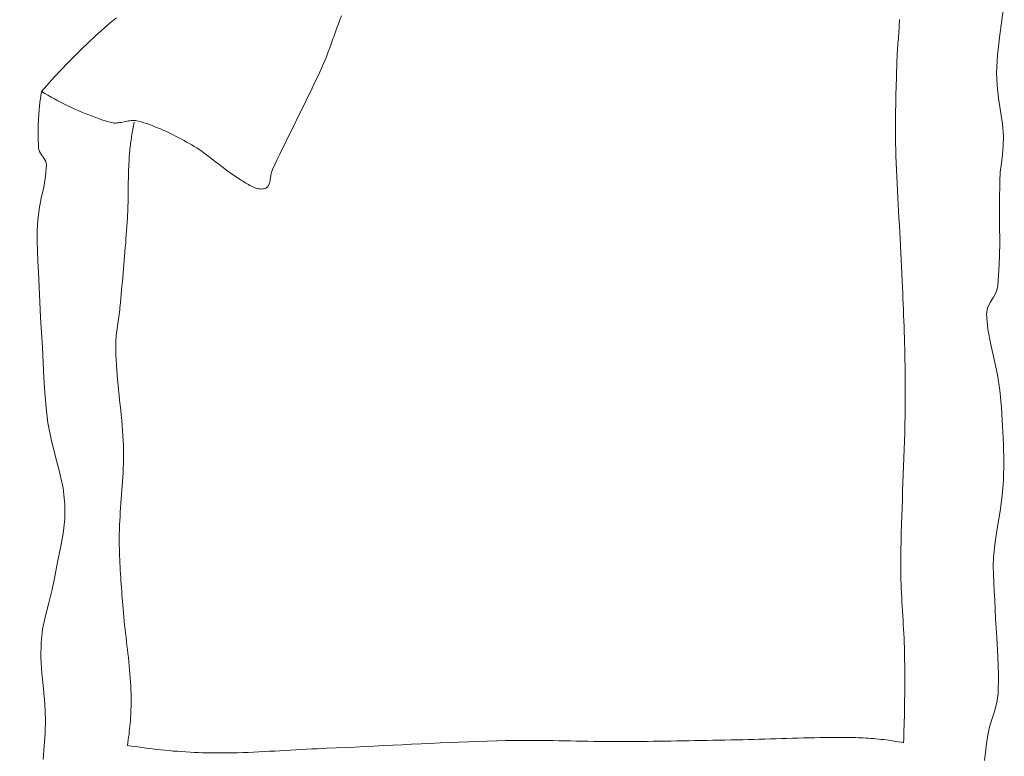
# Model space of a CAD drawing. Units: inches. Extents: x 1484 to 2008, y 1843 to 2590.
# Tile 13 of 21: x 1802 to 1862, y 2126 to 2172. Entities that reach past the tile are written whole.
import ezdxf

# ---------------------------------------------------------------- set-up
doc = ezdxf.new("R2010")
doc.units = ezdxf.units.IN
doc.layers.add('A-ANNO-DIMS', color=2, linetype='Continuous', lineweight=18)
doc.layers.add('A-FURN', color=8, linetype='Continuous', lineweight=18)
doc.styles.get("Standard").update_dxf_attribs({"font": 'arial.ttf'})
doc.dimstyles.new('ISO-25', dxfattribs={"dimtxt": 7, "dimasz": 2.5, "dimexe": 1.25, "dimexo": 0.625, "dimtad": 1, "dimdec": 0, "dimlunit": 3, "dimtxsty": 'Standard', "dimcen": 2.5, "dimadec": 0, "dimazin": 0, "dimtfac": 1, "dimtdec": 0, "dimtmove": 0, "dimatfit": 3, "dimfxl": 1, "dimarcsym": 0})

# ---------------------------------------------------------------- blocks, each defined once
blk = doc.blocks.new('BED-DOUBLE')
for p, q in [((59.548, 52.555), (59.695, 53.637)), ((4.496, 52.387), (3.604, 51.587)), ((4.899, 52.699), (4.496, 52.387)), ((18.499, 52.08), (18.59, 52.327)), ((18.59, 52.327), (18.683, 52.572)), ((18.683, 52.572), (18.778, 52.816)), ((53.205, 52.138), (53.211, 52.285)), ((53.211, 52.285), (53.216, 52.432)), ((53.216, 52.432), (53.22, 52.579)), ((59.397, 51.474), (59.548, 52.555)), ((18.322, 51.584), (18.41, 51.832)), ((18.41, 51.832), (18.499, 52.08)), ((53.167, 51.551), (53.178, 51.698)), ((53.178, 51.698), (53.188, 51.844)), ((53.188, 51.844), (53.197, 51.991)), ((53.197, 51.991), (53.205, 52.138)), ((3.604, 51.587), (2.733, 50.763)), ((18.055, 50.84), (18.145, 51.088)), ((18.145, 51.088), (18.234, 51.336)), ((18.234, 51.336), (18.322, 51.584)), ((53.121, 50.964), (53.133, 51.111)), ((53.133, 51.111), (53.144, 51.257)), ((53.144, 51.257), (53.156, 51.404)), ((53.156, 51.404), (53.167, 51.551)), ((59.275, 50.39), (59.397, 51.474)), ((2.733, 50.763), (1.886, 49.914)), ((17.87, 50.349), (17.964, 50.594)), ((17.964, 50.594), (18.055, 50.84)), ((53.08, 50.377), (53.089, 50.523)), ((53.089, 50.523), (53.099, 50.67)), ((53.099, 50.67), (53.11, 50.817)), ((53.11, 50.817), (53.121, 50.964)), ((1.886, 49.914), (1.063, 49.042)), ((17.565, 49.623), (17.671, 49.863)), ((17.671, 49.863), (17.772, 50.105)), ((17.772, 50.105), (17.87, 50.349)), ((53.054, 49.669), (53.061, 49.936)), ((53.061, 49.936), (53.066, 50.083)), ((53.066, 50.083), (53.072, 50.23)), ((53.072, 50.23), (53.08, 50.377)), ((59.215, 49.303), (59.275, 50.39)), ((17.272, 48.988), (17.419, 49.305)), ((17.419, 49.305), (17.565, 49.623)), ((53.038, 49.135), (53.046, 49.402)), ((53.046, 49.402), (53.054, 49.669)), ((59.246, 48.512), (59.215, 49.303)), ((1.063, 49.042), (0.265, 48.148)), ((16.973, 48.355), (17.123, 48.671)), ((17.123, 48.671), (17.272, 48.988)), ((53.023, 48.601), (53.031, 48.868)), ((53.031, 48.868), (53.038, 49.135)), ((0.265, 48.148), (0.164, 47.454)), ((0.265, 48.148), (0.464, 48.028)), ((0.464, 48.028), (0.665, 47.91)), ((16.669, 47.725), (16.821, 48.04)), ((16.821, 48.04), (16.973, 48.355)), ((53.003, 47.799), (53.009, 48.067)), ((53.009, 48.067), (53.016, 48.334)), ((53.016, 48.334), (53.023, 48.601)), ((59.343, 47.724), (59.246, 48.512)), ((0.164, 47.454), (0.095, 46.755)), ((0.665, 47.91), (0.867, 47.795)), ((0.867, 47.795), (1.07, 47.682)), ((1.07, 47.682), (1.275, 47.572)), ((1.275, 47.572), (1.482, 47.465)), ((1.482, 47.465), (1.69, 47.36)), ((16.362, 47.096), (16.516, 47.41)), ((16.516, 47.41), (16.669, 47.725)), ((52.992, 47.265), (52.997, 47.532)), ((52.997, 47.532), (53.003, 47.799)), ((59.467, 46.937), (59.343, 47.724)), ((1.69, 47.36), (1.899, 47.258)), ((1.899, 47.258), (2.11, 47.158)), ((2.11, 47.158), (2.322, 47.061)), ((2.322, 47.061), (2.535, 46.966)), ((2.535, 46.966), (2.749, 46.875)), ((2.749, 46.875), (2.964, 46.786)), ((16.208, 46.781), (16.362, 47.096)), ((52.983, 46.731), (52.987, 46.998)), ((52.987, 46.998), (52.992, 47.265)), ((59.579, 46.149), (59.467, 46.937)), ((0.095, 46.755), (0.059, 46.053)), ((2.964, 46.786), (3.18, 46.699)), ((3.18, 46.699), (3.398, 46.616)), ((3.398, 46.616), (3.616, 46.535)), ((3.616, 46.535), (3.835, 46.457)), ((3.835, 46.457), (4.055, 46.382)), ((4.055, 46.382), (4.276, 46.31)), ((4.276, 46.31), (4.498, 46.24)), ((4.498, 46.24), (4.581, 46.219)), ((4.581, 46.219), (4.666, 46.205)), ((4.666, 46.205), (4.752, 46.198)), ((4.752, 46.198), (4.839, 46.197)), ((4.839, 46.197), (4.926, 46.202)), ((4.926, 46.202), (5.014, 46.211)), ((5.014, 46.211), (5.102, 46.223)), ((5.102, 46.223), (5.191, 46.238)), ((5.191, 46.238), (5.279, 46.254)), ((5.279, 46.254), (5.368, 46.272)), ((5.368, 46.272), (5.457, 46.29)), ((5.457, 46.29), (5.546, 46.307)), ((5.546, 46.307), (5.635, 46.322)), ((5.635, 46.322), (5.723, 46.335)), ((5.723, 46.335), (5.811, 46.345)), ((5.811, 46.345), (5.899, 46.351)), ((5.899, 46.351), (5.986, 46.352)), ((5.989, 46.252), (5.966, 46.142)), ((5.986, 46.352), (6.072, 46.347)), ((6.072, 46.347), (6.158, 46.335)), ((6.158, 46.335), (6.242, 46.316)), ((6.242, 46.316), (6.416, 46.266)), ((6.416, 46.266), (6.588, 46.213)), ((6.588, 46.213), (6.76, 46.157)), ((15.898, 46.154), (16.053, 46.467)), ((16.053, 46.467), (16.208, 46.781)), ((52.978, 45.93), (52.979, 46.197)), ((52.979, 46.197), (52.981, 46.464)), ((52.981, 46.464), (52.983, 46.731)), ((0.059, 46.053), (0.056, 45.35)), ((5.864, 45.592), (5.846, 45.481)), ((5.883, 45.702), (5.864, 45.592)), ((5.903, 45.812), (5.883, 45.702)), ((5.923, 45.923), (5.903, 45.812)), ((5.944, 46.032), (5.923, 45.923)), ((5.966, 46.142), (5.944, 46.032)), ((6.76, 46.157), (6.931, 46.097)), ((6.931, 46.097), (7.1, 46.035)), ((7.1, 46.035), (7.269, 45.97)), ((7.269, 45.97), (7.437, 45.903)), ((7.437, 45.903), (7.604, 45.833)), ((7.604, 45.833), (7.77, 45.76)), ((7.77, 45.76), (7.935, 45.686)), ((7.935, 45.686), (8.1, 45.609)), ((8.1, 45.609), (8.263, 45.53)), ((15.589, 45.526), (15.743, 45.84)), ((15.743, 45.84), (15.898, 46.154)), ((52.978, 45.663), (52.978, 45.93)), ((52.98, 45.396), (52.978, 45.663)), ((59.64, 45.358), (59.579, 46.149)), ((0.056, 45.35), (0.087, 44.65)), ((5.782, 45.038), (5.767, 44.927)), ((5.797, 45.149), (5.782, 45.038)), ((5.812, 45.26), (5.797, 45.149)), ((5.829, 45.371), (5.812, 45.26)), ((5.846, 45.481), (5.829, 45.371)), ((8.263, 45.53), (8.426, 45.45)), ((8.426, 45.45), (8.587, 45.368)), ((8.587, 45.368), (8.748, 45.284)), ((8.748, 45.284), (8.908, 45.199)), ((8.908, 45.199), (9.068, 45.113)), ((9.068, 45.113), (9.226, 45.025)), ((9.226, 45.025), (9.384, 44.936)), ((15.28, 44.897), (15.434, 45.212)), ((15.434, 45.212), (15.589, 45.526)), ((52.983, 45.129), (52.98, 45.396)), ((52.987, 44.862), (52.983, 45.129)), ((59.63, 44.809), (59.64, 45.358)), ((0.087, 44.65), (0.148, 44.431)), ((0.148, 44.431), (0.271, 44.228)), ((5.707, 44.371), (5.697, 44.259)), ((5.718, 44.482), (5.707, 44.371)), ((5.729, 44.593), (5.718, 44.482)), ((5.741, 44.705), (5.729, 44.593)), ((5.754, 44.816), (5.741, 44.705)), ((5.767, 44.927), (5.754, 44.816)), ((9.384, 44.936), (9.541, 44.847)), ((9.541, 44.847), (9.699, 44.754)), ((9.699, 44.754), (9.854, 44.656)), ((9.854, 44.656), (10.007, 44.555)), ((10.007, 44.555), (10.158, 44.451)), ((10.158, 44.451), (10.307, 44.345)), ((14.974, 44.268), (15.127, 44.583)), ((15.127, 44.583), (15.28, 44.897)), ((52.993, 44.595), (52.987, 44.862)), ((53.005, 44.167), (52.993, 44.595)), ((59.581, 44.261), (59.63, 44.809)), ((0.271, 44.228), (0.412, 44.029)), ((0.412, 44.029), (0.528, 43.826)), ((0.528, 43.826), (0.574, 43.607)), ((5.668, 43.852), (5.658, 43.667)), ((5.68, 44.036), (5.668, 43.852)), ((5.688, 44.148), (5.68, 44.036)), ((5.697, 44.259), (5.688, 44.148)), ((10.307, 44.345), (10.455, 44.236)), ((10.455, 44.236), (10.602, 44.125)), ((10.602, 44.125), (10.748, 44.013)), ((10.748, 44.013), (10.893, 43.9)), ((10.893, 43.9), (11.037, 43.786)), ((11.037, 43.786), (11.182, 43.672)), ((14.671, 43.637), (14.822, 43.953)), ((14.822, 43.953), (14.974, 44.268)), ((53.02, 43.74), (53.005, 44.167)), ((59.514, 43.714), (59.581, 44.261)), ((0.574, 43.607), (0.52, 42.921)), ((5.643, 43.298), (5.637, 43.113)), ((5.65, 43.483), (5.643, 43.298)), ((5.658, 43.667), (5.65, 43.483)), ((11.182, 43.672), (11.327, 43.559)), ((11.327, 43.559), (11.472, 43.446)), ((11.472, 43.446), (11.619, 43.334)), ((11.619, 43.334), (11.766, 43.224)), ((11.766, 43.224), (11.914, 43.116)), ((14.459, 43.134), (14.476, 43.199)), ((14.476, 43.199), (14.497, 43.262)), ((14.497, 43.262), (14.522, 43.32)), ((14.522, 43.32), (14.671, 43.637)), ((53.036, 43.313), (53.02, 43.74)), ((53.055, 42.886), (53.036, 43.313)), ((59.41, 42.617), (59.45, 43.166)), ((59.45, 43.166), (59.514, 43.714)), ((0.52, 42.921), (0.401, 42.241)), ((5.626, 42.559), (5.624, 42.374)), ((5.629, 42.744), (5.626, 42.559)), ((5.633, 42.929), (5.629, 42.744)), ((5.637, 43.113), (5.633, 42.929)), ((11.914, 43.116), (12.064, 43.01)), ((12.064, 43.01), (12.216, 42.907)), ((12.216, 42.907), (12.37, 42.807)), ((12.37, 42.807), (12.526, 42.712)), ((12.526, 42.712), (12.597, 42.669)), ((12.597, 42.669), (12.668, 42.624)), ((12.668, 42.624), (12.741, 42.578)), ((12.741, 42.578), (12.814, 42.532)), ((14.341, 42.509), (14.358, 42.574)), ((14.358, 42.574), (14.372, 42.642)), ((14.372, 42.642), (14.385, 42.711)), ((14.385, 42.711), (14.396, 42.782)), ((14.396, 42.782), (14.407, 42.853)), ((14.407, 42.853), (14.418, 42.925)), ((14.418, 42.925), (14.43, 42.996)), ((14.43, 42.996), (14.443, 43.066)), ((14.443, 43.066), (14.459, 43.134)), ((53.075, 42.458), (53.055, 42.886)), ((59.389, 41.324), (59.41, 42.617)), ((0.401, 42.241), (0.255, 41.563)), ((5.619, 42.005), (5.617, 41.82)), ((5.621, 42.189), (5.619, 42.005)), ((5.624, 42.374), (5.621, 42.189)), ((12.814, 42.532), (12.889, 42.485)), ((12.889, 42.485), (12.964, 42.439)), ((12.964, 42.439), (13.04, 42.394)), ((13.04, 42.394), (13.116, 42.35)), ((13.116, 42.35), (13.194, 42.309)), ((13.194, 42.309), (13.271, 42.27)), ((13.271, 42.27), (13.349, 42.234)), ((13.349, 42.234), (13.427, 42.203)), ((13.427, 42.203), (13.506, 42.176)), ((13.506, 42.176), (13.585, 42.153)), ((13.585, 42.153), (13.663, 42.137)), ((13.663, 42.137), (13.742, 42.126)), ((13.742, 42.126), (13.821, 42.122)), ((13.821, 42.122), (13.899, 42.125)), ((13.899, 42.125), (13.978, 42.136)), ((13.978, 42.136), (14.056, 42.155)), ((14.056, 42.155), (14.112, 42.178)), ((14.112, 42.178), (14.161, 42.208)), ((14.161, 42.208), (14.204, 42.244)), ((14.204, 42.244), (14.241, 42.287)), ((14.241, 42.287), (14.272, 42.336)), ((14.272, 42.336), (14.299, 42.389)), ((14.299, 42.389), (14.322, 42.447)), ((14.322, 42.447), (14.341, 42.509)), ((53.096, 42.031), (53.075, 42.458)), ((53.119, 41.604), (53.096, 42.031)), ((0.255, 41.563), (0.119, 40.884)), ((5.612, 41.45), (5.608, 41.265)), ((5.615, 41.635), (5.612, 41.45)), ((5.617, 41.82), (5.615, 41.635)), ((53.142, 41.177), (53.119, 41.604)), ((0.119, 40.884), (0.031, 40.199)), ((5.598, 40.896), (5.591, 40.711)), ((5.604, 41.081), (5.598, 40.896)), ((5.608, 41.265), (5.604, 41.081)), ((53.166, 40.75), (53.142, 41.177)), ((53.191, 40.323), (53.166, 40.75)), ((59.4, 40.03), (59.389, 41.324)), ((0.031, 40.199), (0.001, 39.561)), ((5.572, 40.342), (5.556, 40.079)), ((5.582, 40.527), (5.572, 40.342)), ((5.591, 40.711), (5.582, 40.527)), ((53.216, 39.896), (53.191, 40.323)), ((0.001, 39.561), (0, 38.922)), ((5.52, 39.554), (5.502, 39.291)), ((5.539, 39.816), (5.52, 39.554)), ((5.556, 40.079), (5.539, 39.816)), ((53.241, 39.469), (53.216, 39.896)), ((59.41, 38.736), (59.4, 40.03)), ((0, 38.922), (0.02, 38.282)), ((5.482, 39.028), (5.462, 38.766)), ((5.502, 39.291), (5.482, 39.028)), ((53.266, 39.043), (53.241, 39.469)), ((53.29, 38.616), (53.266, 39.043)), ((5.441, 38.503), (5.419, 38.24)), ((5.462, 38.766), (5.441, 38.503)), ((53.314, 38.189), (53.29, 38.616)), ((59.388, 37.444), (59.41, 38.736)), ((0.02, 38.282), (0.048, 37.643)), ((5.375, 37.715), (5.352, 37.453)), ((5.397, 37.978), (5.375, 37.715)), ((5.419, 38.24), (5.397, 37.978)), ((53.337, 37.761), (53.314, 38.189)), ((53.359, 37.334), (53.337, 37.761)), ((0.048, 37.643), (0.075, 37.003)), ((5.329, 37.191), (5.306, 36.928)), ((5.352, 37.453), (5.329, 37.191)), ((53.379, 36.907), (53.359, 37.334)), ((59.304, 36.155), (59.388, 37.444)), ((0.075, 37.003), (0.114, 36.068)), ((5.282, 36.666), (5.258, 36.403)), ((5.306, 36.928), (5.282, 36.666)), ((53.398, 36.48), (53.379, 36.907)), ((53.415, 36.053), (53.398, 36.48)), ((0.114, 36.068), (0.158, 35.133)), ((5.211, 35.879), (5.187, 35.616)), ((5.234, 36.141), (5.211, 35.879)), ((5.258, 36.403), (5.234, 36.141)), ((53.429, 35.707), (53.415, 36.053)), ((59.207, 35.794), (59.304, 36.155)), ((5.163, 35.354), (5.14, 35.091)), ((5.187, 35.616), (5.163, 35.354)), ((53.442, 35.361), (53.429, 35.707)), ((53.455, 35.016), (53.442, 35.361)), ((58.829, 35.114), (59.029, 35.451)), ((59.029, 35.451), (59.207, 35.794)), ((0.158, 35.133), (0.209, 34.198)), ((5.093, 34.66), (5.075, 34.517)), ((5.11, 34.804), (5.093, 34.66)), ((5.126, 34.948), (5.11, 34.804)), ((5.14, 35.091), (5.126, 34.948)), ((53.468, 34.67), (53.455, 35.016)), ((53.481, 34.324), (53.468, 34.67)), ((58.605, 34.408), (58.668, 34.77)), ((58.668, 34.77), (58.829, 35.114)), ((0.209, 34.198), (0.263, 33.264)), ((5.015, 34.086), (4.994, 33.943)), ((5.035, 34.23), (5.015, 34.086)), ((5.055, 34.373), (5.035, 34.23)), ((5.075, 34.517), (5.055, 34.373)), ((53.493, 33.978), (53.481, 34.324)), ((58.684, 33.462), (58.605, 34.408)), ((4.935, 33.512), (4.917, 33.369)), ((4.954, 33.656), (4.935, 33.512)), ((4.974, 33.799), (4.954, 33.656)), ((4.994, 33.943), (4.974, 33.799)), ((53.506, 33.632), (53.493, 33.978)), ((53.517, 33.287), (53.506, 33.632)), ((58.854, 32.525), (58.684, 33.462)), ((0.263, 33.264), (0.321, 32.329)), ((4.872, 32.938), (4.862, 32.794)), ((4.885, 33.081), (4.872, 32.938)), ((4.9, 33.225), (4.885, 33.081)), ((4.917, 33.369), (4.9, 33.225)), ((53.528, 32.941), (53.517, 33.287)), ((53.538, 32.595), (53.528, 32.941)), ((0.321, 32.329), (0.373, 31.4)), ((4.848, 32.506), (4.846, 32.361)), ((4.846, 32.361), (4.847, 32.217)), ((4.847, 32.217), (4.856, 31.904)), ((4.854, 32.65), (4.848, 32.506)), ((4.862, 32.794), (4.854, 32.65)), ((53.548, 32.249), (53.538, 32.595)), ((53.556, 31.903), (53.548, 32.249)), ((59.066, 31.592), (58.854, 32.525)), ((4.856, 31.904), (4.87, 31.591)), ((53.564, 31.557), (53.556, 31.903)), ((0.373, 31.4), (0.421, 30.47)), ((4.87, 31.591), (4.888, 31.278)), ((4.888, 31.278), (4.91, 30.965)), ((53.571, 31.211), (53.564, 31.557)), ((53.576, 30.865), (53.571, 31.211)), ((59.269, 30.657), (59.066, 31.592)), ((0.421, 30.47), (0.477, 29.541)), ((4.91, 30.965), (4.935, 30.653)), ((4.935, 30.653), (4.963, 30.341)), ((53.58, 30.52), (53.576, 30.865)), ((53.583, 30.174), (53.58, 30.52)), ((59.412, 29.714), (59.269, 30.657)), ((4.963, 30.341), (4.993, 30.028)), ((4.993, 30.028), (5.024, 29.716)), ((53.585, 29.828), (53.583, 30.174)), ((53.585, 29.482), (53.585, 29.828)), ((0.477, 29.541), (0.554, 28.614)), ((5.024, 29.716), (5.057, 29.404)), ((5.057, 29.404), (5.09, 29.092)), ((53.584, 29.136), (53.585, 29.482)), ((59.514, 28.605), (59.412, 29.714)), ((0.554, 28.614), (0.665, 27.691)), ((5.09, 29.092), (5.123, 28.78)), ((5.123, 28.78), (5.155, 28.468)), ((53.571, 28.107), (53.579, 28.621)), ((53.579, 28.621), (53.584, 29.136)), ((59.594, 27.492), (59.514, 28.605)), ((5.155, 28.468), (5.186, 28.156)), ((5.186, 28.156), (5.216, 27.843)), ((53.561, 27.592), (53.571, 28.107)), ((0.665, 27.691), (0.86, 26.677)), ((5.216, 27.843), (5.243, 27.531)), ((5.243, 27.531), (5.268, 27.219)), ((53.548, 27.078), (53.561, 27.592)), ((59.646, 26.378), (59.594, 27.492)), ((5.268, 27.219), (5.289, 26.906)), ((5.289, 26.906), (5.307, 26.593)), ((53.533, 26.563), (53.548, 27.078)), ((0.86, 26.677), (1.116, 25.673)), ((5.307, 26.593), (5.32, 26.28)), ((5.32, 26.28), (5.329, 25.967)), ((53.516, 26.049), (53.533, 26.563)), ((59.665, 25.264), (59.646, 26.378)), ((1.116, 25.673), (1.379, 24.67)), ((5.329, 25.967), (5.332, 25.696)), ((5.332, 25.696), (5.33, 25.425)), ((53.48, 25.02), (53.499, 25.534)), ((53.499, 25.534), (53.516, 26.049)), ((5.324, 25.155), (5.315, 24.884)), ((5.33, 25.425), (5.324, 25.155)), ((53.46, 24.505), (53.48, 25.02)), ((59.646, 24.15), (59.665, 25.264)), ((1.379, 24.67), (1.595, 23.662)), ((5.288, 24.343), (5.271, 24.073)), ((5.303, 24.614), (5.288, 24.343)), ((5.315, 24.884), (5.303, 24.614)), ((53.441, 23.991), (53.46, 24.505)), ((5.252, 23.802), (5.232, 23.532)), ((5.271, 24.073), (5.252, 23.802)), ((53.421, 23.477), (53.441, 23.991)), ((59.572, 23.194), (59.646, 24.15)), ((1.595, 23.662), (1.71, 22.641)), ((5.212, 23.261), (5.191, 22.991)), ((5.232, 23.532), (5.212, 23.261)), ((53.402, 22.962), (53.421, 23.477)), ((59.44, 22.243), (59.572, 23.194)), ((1.71, 22.641), (1.697, 21.749)), ((5.17, 22.72), (5.15, 22.45)), ((5.191, 22.991), (5.17, 22.72)), ((53.384, 22.448), (53.402, 22.962)), ((5.113, 21.909), (5.098, 21.638)), ((5.131, 22.179), (5.113, 21.909)), ((5.15, 22.45), (5.131, 22.179)), ((53.351, 21.419), (53.367, 21.933)), ((53.367, 21.933), (53.384, 22.448)), ((59.285, 21.294), (59.44, 22.243)), ((1.697, 21.749), (1.596, 20.86)), ((5.085, 21.368), (5.075, 21.097)), ((5.098, 21.638), (5.085, 21.368)), ((53.337, 20.905), (53.351, 21.419)), ((59.14, 20.344), (59.285, 21.294)), ((1.596, 20.86), (1.44, 19.975)), ((5.068, 20.826), (5.065, 20.555)), ((5.075, 21.097), (5.068, 20.826)), ((53.326, 20.39), (53.337, 20.905)), ((5.065, 20.555), (5.066, 20.338)), ((5.066, 20.338), (5.068, 20.12)), ((5.068, 20.12), (5.072, 19.903)), ((53.317, 19.876), (53.326, 20.39)), ((59.037, 19.39), (59.14, 20.344)), ((1.44, 19.975), (1.262, 19.091)), ((5.072, 19.903), (5.078, 19.685)), ((5.078, 19.685), (5.085, 19.468)), ((5.085, 19.468), (5.094, 19.251)), ((53.31, 19.361), (53.317, 19.876)), ((1.262, 19.091), (1.093, 18.209)), ((5.094, 19.251), (5.104, 19.033)), ((5.104, 19.033), (5.115, 18.816)), ((53.307, 18.846), (53.31, 19.361)), ((53.308, 18.568), (53.307, 18.846)), ((59.016, 18.863), (59.037, 19.39)), ((59.023, 18.336), (59.016, 18.863)), ((5.115, 18.816), (5.127, 18.599)), ((5.127, 18.599), (5.141, 18.382)), ((5.141, 18.382), (5.155, 18.164)), ((53.312, 18.29), (53.308, 18.568)), ((53.318, 18.011), (53.312, 18.29)), ((59.048, 17.809), (59.023, 18.336)), ((1.093, 18.209), (0.922, 17.393)), ((5.155, 18.164), (5.17, 17.947)), ((5.17, 17.947), (5.186, 17.73)), ((5.186, 17.73), (5.202, 17.513)), ((53.327, 17.733), (53.318, 18.011)), ((53.338, 17.455), (53.327, 17.733)), ((59.077, 17.282), (59.048, 17.809)), ((0.922, 17.393), (0.715, 16.583)), ((5.202, 17.513), (5.218, 17.296)), ((5.218, 17.296), (5.235, 17.079)), ((5.235, 17.079), (5.252, 16.862)), ((53.35, 17.177), (53.338, 17.455)), ((53.364, 16.899), (53.35, 17.177)), ((59.101, 16.755), (59.077, 17.282)), ((0.715, 16.583), (0.509, 15.773)), ((5.252, 16.862), (5.269, 16.645)), ((5.269, 16.645), (5.286, 16.428)), ((5.286, 16.428), (5.303, 16.211)), ((53.379, 16.62), (53.364, 16.899)), ((53.395, 16.342), (53.379, 16.62)), ((59.156, 15.595), (59.101, 16.755)), ((5.303, 16.211), (5.324, 15.959)), ((5.324, 15.959), (5.346, 15.707)), ((53.412, 16.064), (53.395, 16.342)), ((53.429, 15.786), (53.412, 16.064)), ((0.509, 15.773), (0.338, 14.959)), ((5.346, 15.707), (5.371, 15.456)), ((5.371, 15.456), (5.398, 15.204)), ((5.398, 15.204), (5.426, 14.953)), ((53.445, 15.508), (53.429, 15.786)), ((53.462, 15.23), (53.445, 15.508)), ((53.477, 14.952), (53.462, 15.23)), ((59.229, 14.436), (59.156, 15.595)), ((0.338, 14.959), (0.237, 14.135)), ((5.426, 14.953), (5.454, 14.702)), ((5.454, 14.702), (5.484, 14.451)), ((53.492, 14.674), (53.477, 14.952)), ((53.506, 14.395), (53.492, 14.674)), ((0.237, 14.135), (0.225, 13.181)), ((5.484, 14.451), (5.514, 14.199)), ((5.514, 14.199), (5.544, 13.948)), ((53.518, 14.117), (53.506, 14.395)), ((53.528, 13.839), (53.518, 14.117)), ((59.295, 13.277), (59.229, 14.436)), ((5.544, 13.948), (5.574, 13.697)), ((5.574, 13.697), (5.603, 13.446)), ((5.603, 13.446), (5.631, 13.195)), ((53.536, 13.561), (53.528, 13.839)), ((53.542, 13.282), (53.536, 13.561)), ((0.225, 13.181), (0.286, 12.227)), ((5.631, 13.195), (5.658, 12.943)), ((5.658, 12.943), (5.684, 12.692)), ((53.545, 13.015), (53.542, 13.282)), ((53.548, 12.748), (53.545, 13.015)), ((59.33, 12.118), (59.295, 13.277)), ((0.286, 12.227), (0.381, 11.273)), ((5.684, 12.692), (5.707, 12.44)), ((5.707, 12.44), (5.729, 12.189)), ((5.729, 12.189), (5.748, 11.937)), ((53.55, 12.481), (53.548, 12.748)), ((53.552, 12.214), (53.55, 12.481)), ((53.553, 11.947), (53.552, 12.214)), ((5.748, 11.937), (5.765, 11.685)), ((5.765, 11.685), (5.778, 11.433)), ((53.552, 11.413), (53.553, 11.68)), ((53.553, 11.68), (53.553, 11.947)), ((59.308, 10.959), (59.33, 12.118)), ((0.381, 11.273), (0.472, 10.318)), ((5.778, 11.433), (5.788, 11.18)), ((5.788, 11.18), (5.793, 11.01)), ((5.793, 11.01), (5.796, 10.839)), ((53.548, 10.878), (53.55, 11.146)), ((53.55, 11.146), (53.552, 11.413)), ((59.238, 10.441), (59.308, 10.959)), ((5.797, 10.498), (5.795, 10.328)), ((5.796, 10.839), (5.797, 10.669)), ((5.797, 10.669), (5.797, 10.498)), ((53.537, 10.077), (53.541, 10.344)), ((53.541, 10.344), (53.545, 10.611)), ((53.545, 10.611), (53.548, 10.878)), ((59.106, 9.932), (59.238, 10.441)), ((0.472, 10.318), (0.518, 9.363)), ((5.78, 9.816), (5.771, 9.646)), ((5.786, 9.987), (5.78, 9.816)), ((5.792, 10.157), (5.786, 9.987)), ((5.795, 10.328), (5.792, 10.157)), ((53.525, 9.543), (53.531, 9.81)), ((53.531, 9.81), (53.537, 10.077)), ((58.945, 9.427), (59.106, 9.932)), ((0.518, 9.363), (0.498, 8.541)), ((5.737, 9.135), (5.722, 8.965)), ((5.75, 9.305), (5.737, 9.135)), ((5.762, 9.475), (5.75, 9.305)), ((5.771, 9.646), (5.762, 9.475)), ((53.511, 9.009), (53.519, 9.276)), ((53.519, 9.276), (53.525, 9.543)), ((58.791, 8.92), (58.945, 9.427)), ((0.498, 8.541), (0.441, 7.719)), ((5.688, 8.625), (5.668, 8.456)), ((5.706, 8.795), (5.688, 8.625)), ((5.722, 8.965), (5.706, 8.795)), ((53.494, 8.475), (53.503, 8.742)), ((53.503, 8.742), (53.511, 9.009)), ((58.678, 8.406), (58.791, 8.92)), ((5.6, 7.949), (5.574, 7.78)), ((5.624, 8.117), (5.6, 7.949)), ((5.647, 8.286), (5.624, 8.117)), ((5.668, 8.456), (5.647, 8.286)), ((23.697, 7.874), (24.281, 7.901)), ((24.281, 7.901), (24.864, 7.927)), ((24.864, 7.927), (25.448, 7.952)), ((25.448, 7.952), (26.031, 7.976)), ((26.031, 7.976), (26.615, 7.998)), ((26.615, 7.998), (27.199, 8.019)), ((27.199, 8.019), (27.783, 8.038)), ((27.783, 8.038), (28.366, 8.055)), ((28.366, 8.055), (28.95, 8.069)), ((28.95, 8.069), (29.311, 8.077)), ((29.311, 8.077), (29.672, 8.081)), ((29.672, 8.081), (30.033, 8.084)), ((30.033, 8.084), (30.394, 8.084)), ((30.394, 8.084), (30.755, 8.083)), ((30.755, 8.083), (31.116, 8.081)), ((31.116, 8.081), (31.477, 8.077)), ((31.477, 8.077), (31.838, 8.072)), ((31.838, 8.072), (32.199, 8.066)), ((32.199, 8.066), (32.56, 8.059)), ((32.56, 8.059), (32.921, 8.053)), ((32.921, 8.053), (33.282, 8.046)), ((33.282, 8.046), (33.643, 8.039)), ((33.643, 8.039), (34.004, 8.033)), ((34.004, 8.033), (34.365, 8.027)), ((34.365, 8.027), (34.725, 8.022)), ((34.725, 8.022), (35.086, 8.018)), ((35.086, 8.018), (35.447, 8.015)), ((35.447, 8.015), (35.808, 8.014)), ((35.808, 8.014), (36.169, 8.014)), ((36.169, 8.014), (36.538, 8.016)), ((36.538, 8.016), (36.907, 8.019)), ((36.907, 8.019), (37.276, 8.022)), ((37.276, 8.022), (37.645, 8.026)), ((37.645, 8.026), (38.014, 8.03)), ((38.014, 8.03), (38.383, 8.035)), ((38.383, 8.035), (38.752, 8.041)), ((38.752, 8.041), (39.121, 8.046)), ((39.121, 8.046), (39.49, 8.053)), ((39.49, 8.053), (39.859, 8.059)), ((39.859, 8.059), (40.228, 8.066)), ((40.228, 8.066), (40.597, 8.073)), ((40.597, 8.073), (40.966, 8.08)), ((40.966, 8.08), (41.335, 8.087)), ((41.335, 8.087), (41.704, 8.094)), ((41.704, 8.094), (42.073, 8.101)), ((42.073, 8.101), (42.442, 8.108)), ((42.442, 8.108), (42.811, 8.115)), ((42.811, 8.115), (43.18, 8.122)), ((43.18, 8.122), (43.549, 8.128)), ((43.549, 8.128), (43.89, 8.135)), ((43.89, 8.135), (44.231, 8.143)), ((44.231, 8.143), (44.572, 8.152)), ((44.572, 8.152), (44.913, 8.161)), ((44.913, 8.161), (45.254, 8.172)), ((45.254, 8.172), (45.595, 8.182)), ((45.595, 8.182), (45.936, 8.193)), ((45.936, 8.193), (46.277, 8.204)), ((46.277, 8.204), (46.618, 8.215)), ((46.618, 8.215), (46.959, 8.226)), ((46.959, 8.226), (47.3, 8.235)), ((47.3, 8.235), (47.64, 8.244)), ((47.64, 8.244), (47.981, 8.252)), ((47.981, 8.252), (48.322, 8.259)), ((48.322, 8.259), (48.663, 8.264)), ((48.663, 8.264), (49.004, 8.268)), ((49.004, 8.268), (49.345, 8.269)), ((49.345, 8.269), (49.686, 8.269)), ((49.686, 8.269), (50.027, 8.266)), ((50.027, 8.266), (50.368, 8.261)), ((50.368, 8.261), (50.524, 8.258)), ((50.524, 8.258), (50.68, 8.253)), ((50.68, 8.253), (50.836, 8.247)), ((50.836, 8.247), (50.992, 8.239)), ((50.992, 8.239), (51.148, 8.23)), ((51.148, 8.23), (51.304, 8.22)), ((51.304, 8.22), (51.46, 8.209)), ((51.46, 8.209), (51.616, 8.196)), ((51.616, 8.196), (51.772, 8.182)), ((51.772, 8.182), (51.928, 8.166)), ((51.928, 8.166), (52.083, 8.15)), ((52.083, 8.15), (52.238, 8.132)), ((52.238, 8.132), (52.394, 8.112)), ((52.394, 8.112), (52.549, 8.092)), ((52.549, 8.092), (52.703, 8.07)), ((52.703, 8.07), (52.858, 8.047)), ((52.858, 8.047), (53.012, 8.022)), ((53.012, 8.022), (53.166, 7.997)), ((53.166, 7.997), (53.32, 7.97)), ((53.32, 7.97), (53.474, 7.941)), ((53.474, 7.941), (53.484, 8.208)), ((53.484, 8.208), (53.494, 8.475)), ((58.598, 7.887), (58.678, 8.406)), ((0.441, 7.719), (0.376, 6.898)), ((5.574, 7.78), (5.829, 7.739)), ((5.829, 7.739), (6.085, 7.7)), ((6.085, 7.7), (6.341, 7.663)), ((6.341, 7.663), (6.598, 7.627)), ((6.598, 7.627), (6.855, 7.593)), ((6.855, 7.593), (7.112, 7.562)), ((7.112, 7.562), (7.369, 7.532)), ((7.369, 7.532), (7.626, 7.504)), ((7.626, 7.504), (7.884, 7.477)), ((7.884, 7.477), (8.142, 7.453)), ((8.142, 7.453), (8.4, 7.43)), ((8.4, 7.43), (8.658, 7.41)), ((8.658, 7.41), (8.917, 7.391)), ((8.917, 7.391), (9.175, 7.374)), ((9.175, 7.374), (9.434, 7.359)), ((9.434, 7.359), (9.692, 7.346)), ((9.692, 7.346), (9.951, 7.335)), ((9.951, 7.335), (10.209, 7.326)), ((10.209, 7.326), (10.468, 7.318)), ((10.468, 7.318), (10.727, 7.313)), ((10.727, 7.313), (11.055, 7.309)), ((11.055, 7.309), (11.382, 7.308)), ((11.382, 7.308), (11.71, 7.31)), ((11.71, 7.31), (12.038, 7.316)), ((12.038, 7.316), (12.365, 7.324)), ((12.365, 7.324), (12.693, 7.334)), ((12.693, 7.334), (13.021, 7.346)), ((13.021, 7.346), (13.348, 7.361)), ((13.348, 7.361), (13.676, 7.376)), ((13.676, 7.376), (14.003, 7.393)), ((14.003, 7.393), (14.331, 7.411)), ((14.331, 7.411), (14.659, 7.43)), ((14.659, 7.43), (14.986, 7.449)), ((14.986, 7.449), (15.314, 7.468)), ((15.314, 7.468), (15.641, 7.487)), ((15.641, 7.487), (15.969, 7.506)), ((15.969, 7.506), (16.296, 7.524)), ((16.296, 7.524), (16.624, 7.541)), ((16.624, 7.541), (16.951, 7.557)), ((16.951, 7.557), (17.279, 7.571)), ((17.279, 7.571), (17.863, 7.596)), ((17.863, 7.596), (18.446, 7.622)), ((18.446, 7.622), (19.03, 7.649)), ((19.03, 7.649), (19.613, 7.676)), ((19.613, 7.676), (20.197, 7.704)), ((20.197, 7.704), (20.78, 7.733)), ((20.78, 7.733), (21.363, 7.761)), ((21.363, 7.761), (21.947, 7.79)), ((21.947, 7.79), (22.53, 7.818)), ((22.53, 7.818), (23.114, 7.846)), ((23.114, 7.846), (23.697, 7.874)), ((58.48, 6.841), (58.527, 7.365)), ((58.527, 7.365), (58.598, 7.887))]:
    blk.add_line(p, q)
blk = doc.blocks.new('*D12')
at = {"layer": 'A-ANNO-DIMS', "color": 0, "lineweight": -2, "transparency": 16777216}
for p, q in [((1798.407, 2117.29), (1798.407, 2180.139)), ((1793.295, 2117.29), (1799.657, 2117.29)), ((1798.407, 2086.463), (1798.407, 2114.79)), ((1793.295, 2083.963), (1799.657, 2083.963))]:
    blk.add_line(p, q, dxfattribs=at)
at = {"layer": 'A-ANNO-DIMS', "color": 0, "transparency": 16777216}
for points in [[(1797.99, 2114.79), (1798.824, 2114.79), (1798.407, 2117.29)], [(1797.99, 2086.463), (1798.824, 2086.463), (1798.407, 2083.963)]]:
    blk.add_solid(points, dxfattribs=at)
at = {"layer": 'Defpoints', "color": 0, "transparency": 16777216}
for p in [(1792.67, 2117.29), (1798.407, 2117.29), (1792.67, 2083.963)]:
    blk.add_point(p, dxfattribs=at)
at = {"layer": 'A-ANNO-DIMS', "color": 0, "transparency": 16777216, "insert": (1794.163, 2149.965), "char_height": 7, "attachment_point": 5, "rotation": 90}
blk.add_mtext('2\'-9 1/2" TYP.', dxfattribs=at)

msp = doc.modelspace()

# ---------------------------------------------------------------- block references
at = {"layer": 'A-FURN'}
msp.add_blockref('BED-DOUBLE', (1802.632, 2119.201), dxfattribs=at)

# ---------------------------------------------------------------- dimensions: what is measured, and where the dimension line sits
at = {"layer": 'A-ANNO-DIMS'}
dim = msp.add_linear_dim(base=(1798.407, 2117.29), p1=(1792.67, 2083.963), p2=(1792.67, 2117.29), angle=90, text='<> TYP.', dimstyle='ISO-25', override={"dimdec": 1, "dimlfac": 1, "dimrnd": 0, "dimzin": 1, "dimdsep": 46, "dimlunit": 4, "dimfrac": 2}, dxfattribs=at)
dim.commit()
dim.dimension.update_dxf_attribs({"geometry": '*D12', "text_midpoint": (1794.163, 2149.965)})

doc.saveas('drawing.dxf')
